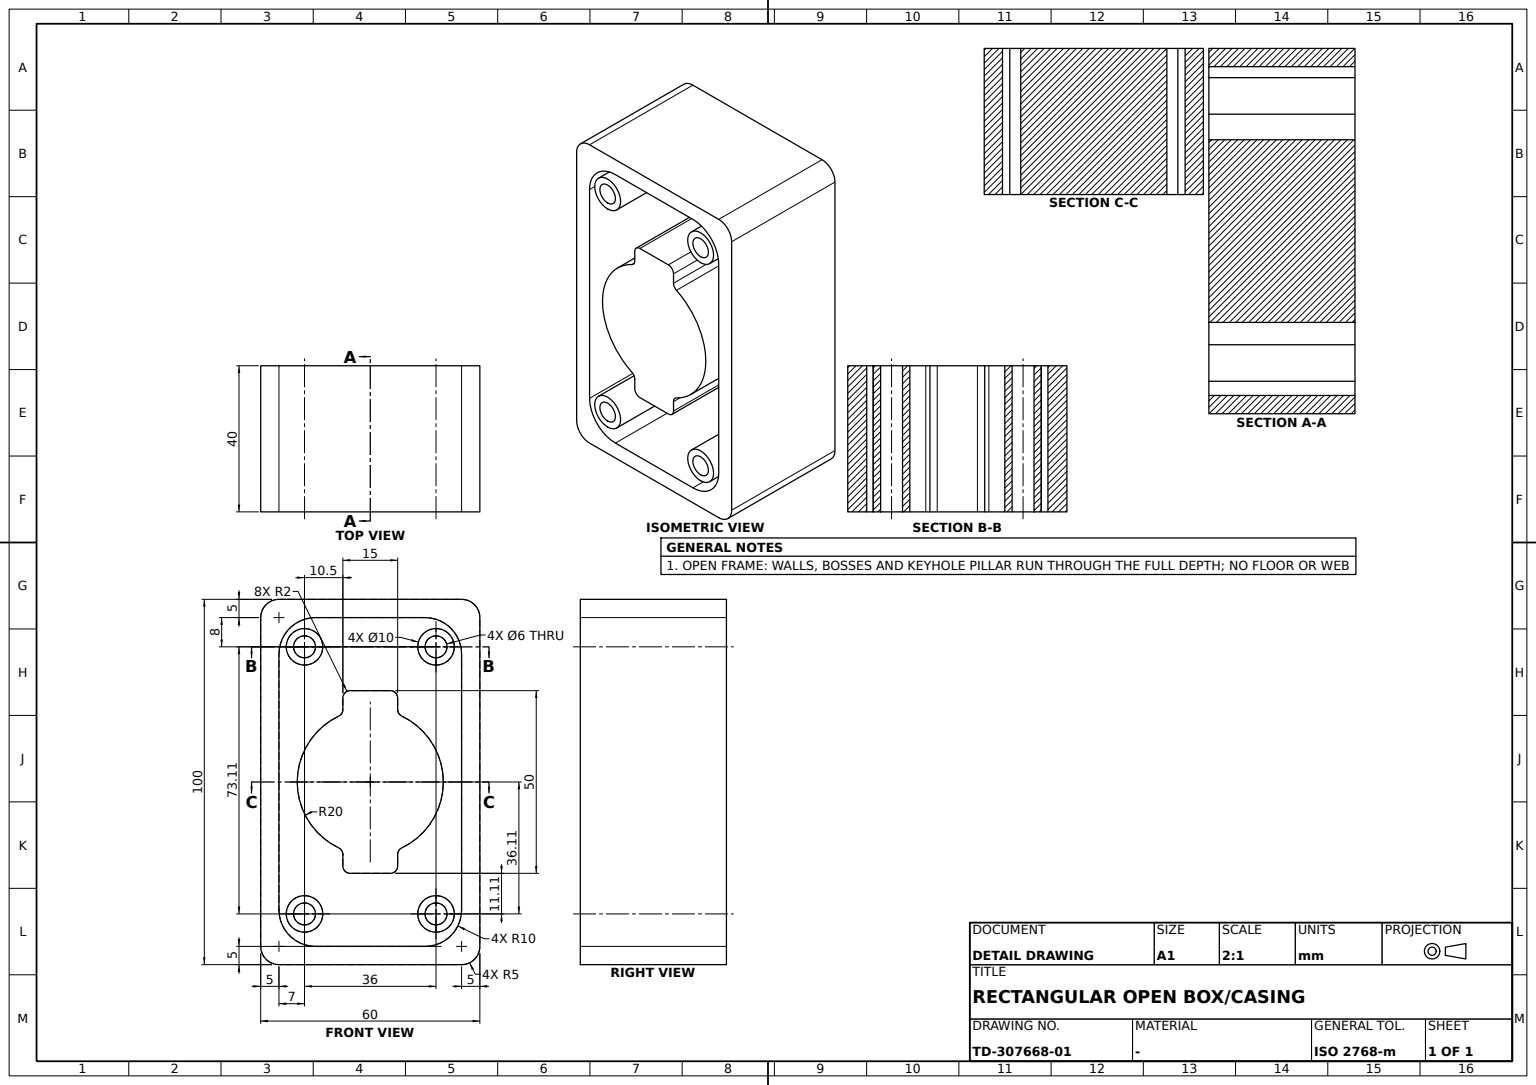
CATIA V5 part; units mm, degrees
sketch "Sketch1" plane through (0, 0, 0) normal (1, 0, 0) x (0, 1, 0)
  line L0 (-30, 50) -> (30, 50)
  line L1 (30, 50) -> (30, -50)
  line L2 (30, -50) -> (-30, -50)
  line L3 (-30, -50) -> (-30, 50)
  line L4 (-25, 45) -> (25, 45)
  line L5 (25, 45) -> (25, -45)
  line L6 (25, -45) -> (-25, -45)
  line L7 (-25, -45) -> (-25, 45)
  circle A0 centre (18, 37) radius 5
  circle A1 centre (18, 37) radius 3
  circle A2 centre (18, -36.1114) radius 5
  point P0 (18, -36.1114)
  circle A3 centre (18, -36.1114) radius 3
  circle A4 centre (-18, 37) radius 5
  point P1 (-18, 37)
  circle A5 centre (-18, 37) radius 3
  circle A6 centre (-18, -36.1114) radius 5
  point P2 (-18, -36.1114)
  circle A7 centre (-18, -36.1114) radius 3
  line L8 (-7.5, 25) -> (7.5, 25)
  line L9 (7.5, 25) -> (7.5, -25)
  line L10 (7.5, -25) -> (-7.5, -25)
  line L11 (-7.5, -25) -> (-7.5, 25)
  dimension "length L1" = 100
  dimension "length L2" = 60
  dimension "distance L5 L1" = 5
  dimension "distance L0 L4" = 5
  dimension "distance L6 L2" = 5
  dimension "distance L7 L3" = 5
  dimension "radius A1" = 3
  dimension "radius A0" = 5
  dimension "radius A3" = 3
  dimension "radius A2" = 5
  dimension "length L9" = 50
  dimension "length L10" = 15
  dimension "distance P1 P2" = 73.1114
  dimension "distance P1 L4" = 8
  dimension "distance P1 L7" = 7
  dimension "distance P0 L5" = 7
  constraint horizontal L0 x-axis
  constraint horizontal L2 x-axis
  constraint horizontal L4 x-axis
  constraint horizontal L6 x-axis
  constraint horizontal L8 x-axis
  constraint horizontal L10 x-axis
  constraint vertical L1 y-axis
  constraint vertical L3 y-axis
  constraint vertical L5 y-axis
  constraint vertical L7 y-axis
  constraint vertical L9 y-axis
  constraint vertical L11 y-axis
  constraint symmetry L0 L2 x-axis
  constraint symmetry L3 L1 y-axis
  constraint symmetry A0 A4 y-axis
  constraint symmetry A1 A5 y-axis
  constraint symmetry A2 A6 y-axis
  constraint symmetry A3 A7 y-axis
  constraint symmetry L8 L10 x-axis
  constraint symmetry L11 L9 y-axis
extrude "Pad1" add sketch "Sketch1" along normal mid plane 40
fillet "Fillet1" radius 10 1 edges at (0, -25, 45)
fillet "Fillet2" radius 10 1 edges at (0, 25, 45)
fillet "Fillet3" radius 10 1 edges at (0, 25, -45)
fillet "Fillet4" radius 10 1 edges at (0, -25, -45)
sketch "Sketch2" plane through (20, 0, 0) normal (1, 0, 0) x (0, 1, 0)
  circle A0 centre (0, 0) radius 20
  dimension "radius A0" = 20
extrude "Pad2" add sketch "Sketch2" against normal blind 40
fillet "Fillet5" radius 5 1 edges at (0, 30, 50)
fillet "Fillet6" radius 5 1 edges at (0, -30, 50)
fillet "Fillet7" radius 5 1 edges at (0, -30, -50)
fillet "Fillet8" radius 5 1 edges at (0, 30, -50)
fillet "Fillet9" radius 2 1 edges at (0, 7.5, 25)
fillet "Fillet10" radius 2 1 edges at (0, -7.5, 25)
fillet "Fillet11" radius 2 1 edges at (0, -7.5, -25)
fillet "Fillet12" radius 2 1 edges at (0, 7.5, -25)
fillet "Fillet13" radius 2 1 edges at (0, -7.5, 18.5405)
fillet "Fillet14" radius 2 1 edges at (0, 7.5, 18.5405)
fillet "Fillet15" radius 2 1 edges at (0, 7.5, -18.5405)
fillet "Fillet16" radius 2 1 edges at (0, -7.5, -18.5405)
